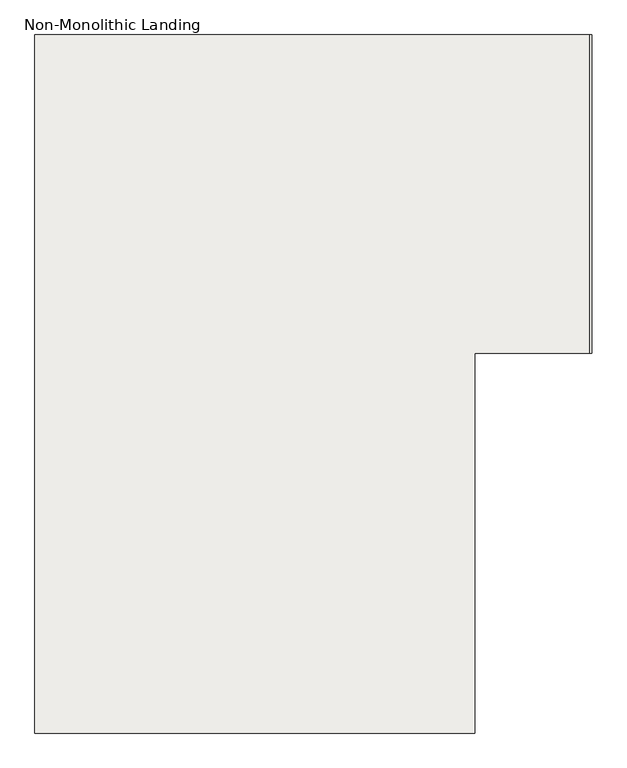
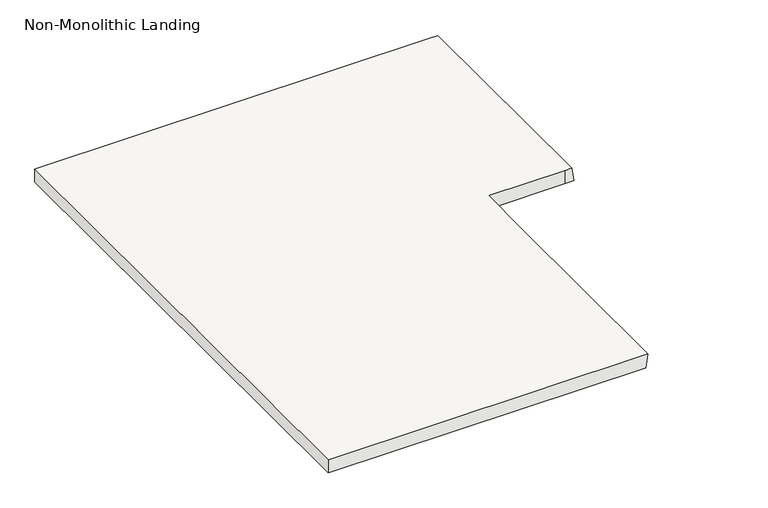
"""IFC4 building model written with IfcOpenShell, lengths in millimetres: slab geometry, Non-Monolithic Landing."""

from ifc_helpers import new_model, si_unit, origin, place, context, project, spatial, faceted_brep, source, transform, mapped, element, save


def non_monolithic_landing_29a5f23a(model_context):
    return source(origin(), model_context, "Body", "Brep", [
        faceted_brep([(-9053.6870075, 2408.8252453, 1565.2173913), (-9046.4995075, 2408.8252453, 1515.2173913), (-9046.4995075, 3244.2865734, 1515.2173913), (-9053.6870075, 3244.2865734, 1565.2173913), (-9353.6870075, 2212.3123547, 1565.2173913), (-9353.6870075, 2408.8252453, 1565.2173913), (-9078.6870075, 2408.8252453, 1565.2173913), (-9078.6870075, 3244.2865734, 1565.2173913), (-10508.0870075, 3244.2865734, 1565.2173913), (-10508.0870075, 1412.2865734, 1565.2173913), (-9353.6870075, 1412.2865734, 1565.2173913), (-9353.6870075, 2408.8252453, 1515.2173913), (-9353.6870075, 2212.3123547, 1515.2173913), (-9360.8745075, 2212.3123547, 1515.2173913), (-9360.8745075, 1412.2865734, 1515.2173913), (-10508.0870075, 1412.2865734, 1515.2173913), (-10508.0870075, 3244.2865734, 1515.2173913), (-9078.6870075, 3244.2865734, 1515.2173913), (-9078.6870075, 2408.8252453, 1515.2173913)], [[[0, 1, 2, 3]], [[4, 5, 6, 0, 3, 7, 8, 9, 10]], [[11, 12, 13, 14, 15, 16, 17, 2, 1, 18]], [[5, 4, 12, 11]], [[6, 5, 11, 18]], [[0, 6, 18, 1]], [[7, 3, 2, 17]], [[8, 7, 17, 16]], [[9, 8, 16, 15]], [[10, 9, 15, 14]], [[4, 13, 12]], [[13, 4, 10, 14]]]),
    ])


if __name__ == "__main__":
    model = new_model("IFC4")
    model_context = context("Model", 3, world=origin())
    ifc_project = project(units=[si_unit("LENGTHUNIT", "METRE", prefix="MILLI")], contexts=[model_context])
    site = spatial("IfcSite", under=ifc_project)
    building = spatial("IfcBuilding", under=site)
    placement = place(None, origin())
    non_monolithic_landing_shape = non_monolithic_landing_29a5f23a(model_context)
    element("IfcSlab", 1, ObjectType="Non-Monolithic Landing", at=placement, inside=building, context=model_context, shape_type="MappedRepresentation", body=[
        mapped(non_monolithic_landing_shape, transform((0.0, 0.0, 0.0), x_axis=(1.0, 0.0, 0.0), y_axis=(0.0, 1.0, 0.0), z_axis=(0.0, 0.0, 1.0))),
    ])
    save(model, "model.ifc")
